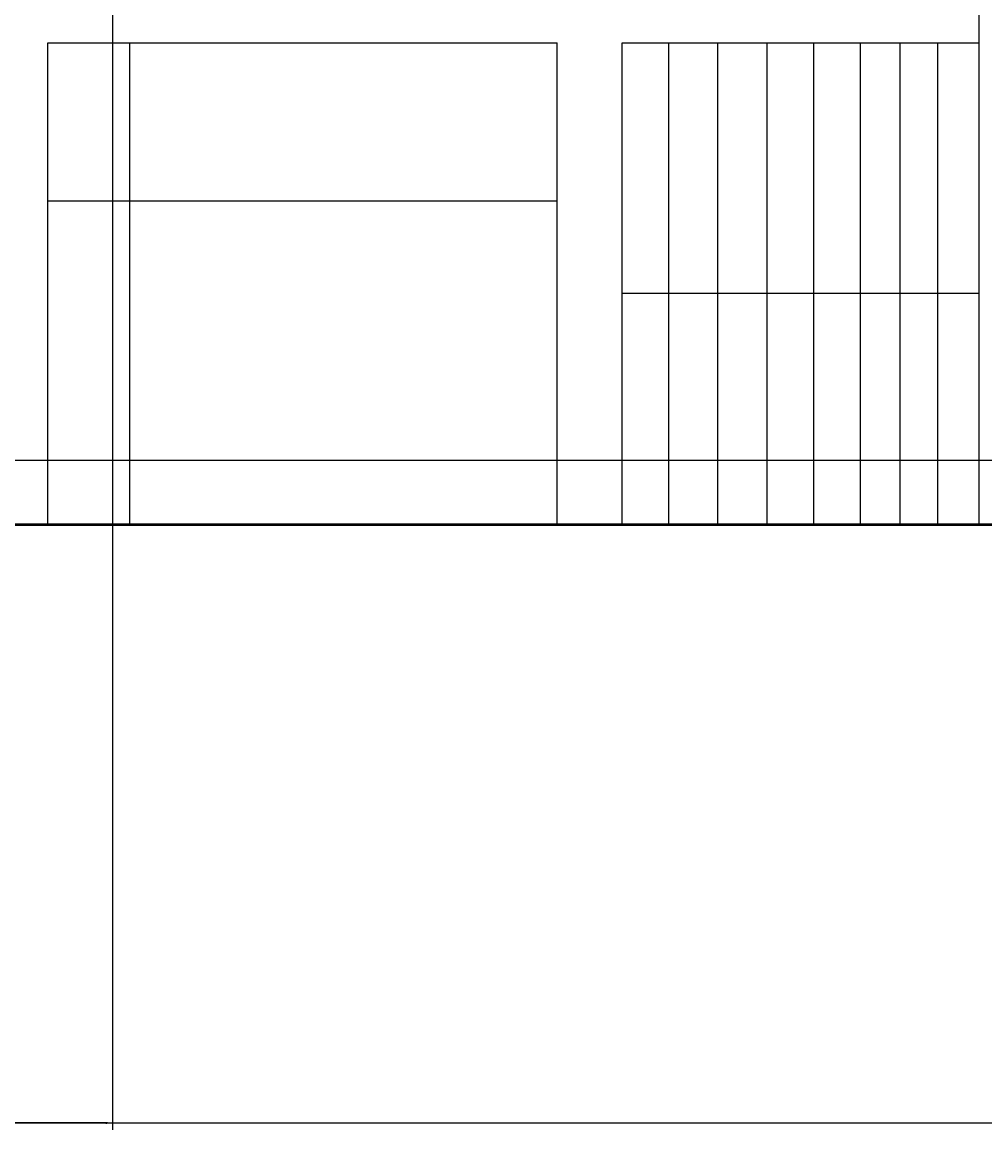
# Model space of a CAD drawing. Units: inches. Extents: x -117 to 121, y -77 to 40.
# Tile 6 of 45: x -48 to -23, y -77 to -48. Entities that reach past the tile are written whole.
import ezdxf

# ---------------------------------------------------------------- set-up
doc = ezdxf.new("R2010")
doc.units = ezdxf.units.IN
doc.header["$MEASUREMENT"] = 0
for name, color, linetype, lineweight in [('A-ANNO-DIMS', 2, 'Continuous', 18), ('A-ELEV', 7, 'Continuous', 25), ('A-ELEV-GRND', 7, 'Continuous', 50)]:
    doc.layers.add(name, color=color, linetype=linetype, lineweight=lineweight)
doc.styles.get("Standard").update_dxf_attribs({"font": 'arial.ttf'})
doc.dimstyles.get("Standard").update_dxf_attribs({"dimtxt": 0.18, "dimasz": 0.18, "dimexe": 0.18, "dimexo": 0.0625, "dimgap": 0.09, "dimtad": 0, "dimtih": 1, "dimtoh": 1, "dimdec": 4, "dimzin": 0, "dimdsep": 46, "dimtxsty": 'Standard', "dimcen": 0.09, "dimadec": 0, "dimazin": 0, "dimtfac": 1, "dimtdec": 4, "dimtofl": 0, "dimtmove": 0, "dimatfit": 3, "dimfxl": 1, "dimtolj": 1, "dimtzin": 0, "dimarcsym": 0})

# ---------------------------------------------------------------- blocks, each defined once
blk = doc.blocks.new('*D7')
at = {"layer": 'A-ANNO-DIMS', "color": 0, "lineweight": -2, "transparency": 16777216}
for p, q in [((-77.763, -61.431), (-77.763, -77.193)), ((90.549, -61.438), (90.549, -77.193)), ((-77.583, -77.013), (6.008, -77.013)), ((90.369, -77.013), (6.778, -77.013))]:
    blk.add_line(p, q, dxfattribs=at)
at = {"layer": 'A-ANNO-DIMS', "color": 0, "transparency": 16777216}
for points in [[(-77.583, -76.983), (-77.583, -77.043), (-77.763, -77.013)], [(90.369, -76.983), (90.369, -77.043), (90.549, -77.013)]]:
    blk.add_solid(points, dxfattribs=at)
at = {"layer": 'Defpoints', "color": 0, "transparency": 16777216}
for p in [(-77.763, -61.369), (90.549, -61.376), (90.549, -77.013)]:
    blk.add_point(p, dxfattribs=at)
at = {"layer": 'A-ANNO-DIMS', "color": 0, "transparency": 16777216, "insert": (6.393, -77.013), "char_height": 0.18, "attachment_point": 5}
blk.add_mtext('\\A1;168.3', dxfattribs=at)
blk = doc.blocks.new('*D13')
at = {"layer": 'A-ANNO-DIMS', "color": 0, "lineweight": -2, "transparency": 16777216}
for p, q in [((-2.663, 27.063), (-117.024, 27.063)), ((-116.844, 26.883), (-116.844, -16.974)), ((-116.844, -61.196), (-116.844, -17.338)), ((-106.096, -61.376), (-117.024, -61.376))]:
    blk.add_line(p, q, dxfattribs=at)
at = {"layer": 'A-ANNO-DIMS', "color": 0, "transparency": 16777216}
for points in [[(-116.874, 26.883), (-116.814, 26.883), (-116.844, 27.063)], [(-116.874, -61.196), (-116.814, -61.196), (-116.844, -61.376)]]:
    blk.add_solid(points, dxfattribs=at)
at = {"layer": 'Defpoints', "color": 0, "transparency": 16777216}
for p in [(-2.6, 27.063), (-116.844, -61.376), (-106.034, -61.376)]:
    blk.add_point(p, dxfattribs=at)
at = {"layer": 'A-ANNO-DIMS', "color": 0, "transparency": 16777216, "insert": (-116.844, -17.156), "char_height": 0.18, "attachment_point": 5}
blk.add_mtext('\\A1;88.44', dxfattribs=at)
blk = doc.blocks.new('*D37')
at = {"layer": 'A-ANNO-DIMS', "color": 0, "lineweight": -2, "transparency": 16777216}
for p, q in [((-3.912, -45.613), (-117.024, -45.613)), ((-116.844, -45.793), (-116.844, -52.47)), ((-116.844, -59.512), (-116.844, -52.834)), ((-3.912, -59.692), (-117.024, -59.692))]:
    blk.add_line(p, q, dxfattribs=at)
at = {"layer": 'A-ANNO-DIMS', "color": 0, "transparency": 16777216}
for points in [[(-116.874, -45.793), (-116.814, -45.793), (-116.844, -45.613)], [(-116.874, -59.512), (-116.814, -59.512), (-116.844, -59.692)]]:
    blk.add_solid(points, dxfattribs=at)
at = {"layer": 'Defpoints', "color": 0, "transparency": 16777216}
for p in [(-116.844, -45.613), (-3.85, -45.613), (-3.85, -59.692)]:
    blk.add_point(p, dxfattribs=at)
at = {"layer": 'A-ANNO-DIMS', "color": 0, "transparency": 16777216, "insert": (-116.844, -52.652), "char_height": 0.18, "attachment_point": 5}
blk.add_mtext('\\A1;14.079', dxfattribs=at)
blk = doc.blocks.new('*D48')
at = {"layer": 'A-ANNO-DIMS', "color": 0, "lineweight": -2, "transparency": 16777216}
for p, q in [((-65.167, -39.778), (-65.167, -77.193)), ((-45.533, -39.778), (-45.533, -77.193)), ((-64.987, -77.013), (-55.805, -77.013)), ((-45.713, -77.013), (-54.895, -77.013))]:
    blk.add_line(p, q, dxfattribs=at)
at = {"layer": 'A-ANNO-DIMS', "color": 0, "transparency": 16777216}
for points in [[(-64.987, -76.983), (-64.987, -77.043), (-65.167, -77.013)], [(-45.713, -76.983), (-45.713, -77.043), (-45.533, -77.013)]]:
    blk.add_solid(points, dxfattribs=at)
at = {"layer": 'Defpoints', "color": 0, "transparency": 16777216}
for p in [(-65.167, -39.716), (-45.533, -39.716), (-45.533, -77.013)]:
    blk.add_point(p, dxfattribs=at)
at = {"layer": 'A-ANNO-DIMS', "color": 0, "transparency": 16777216, "insert": (-55.35, -77.013), "char_height": 0.18, "attachment_point": 5}
blk.add_mtext('\\A1;19.634', dxfattribs=at)

msp = doc.modelspace()

# ---------------------------------------------------------------- linework, layer by layer
at = {"layer": 'A-ELEV'}
for p, q in [((-22.8601, -61.3756), (-22.8601, -31.9617)), ((-47.2265, -61.3756), (-47.2265, -48.7698)), ((-47.2265, -48.7698), (-33.8996, -48.7698)), ((-45.0735, -61.3756), (-45.0735, -48.7698)), ((-33.8996, -61.3756), (-33.8996, -48.7698)), ((-32.195, -61.3756), (-32.195, -48.7698)), ((-32.195, -48.7698), (-22.8601, -48.7698)), ((-30.9878, -48.7698), (-30.9878, -61.3756)), ((-29.7033, -48.7698), (-29.7033, -61.3756)), ((-28.4189, -48.7698), (-28.4189, -61.3756)), ((-27.1956, -48.7698), (-27.1956, -61.3756)), ((-25.9723, -48.7698), (-25.9723, -61.3756)), ((-24.9326, -48.7698), (-24.9326, -61.3756)), ((-23.9539, -48.7698), (-23.9539, -61.3756)), ((-47.2265, -52.905), (-33.8996, -52.905)), ((-32.195, -55.3185), (-22.8601, -55.3185))]:
    msp.add_line(p, q, dxfattribs=at)
at = {"layer": 'A-ELEV-GRND'}
msp.add_line((90.5486, -61.3756), (-87.9273, -61.3756), dxfattribs=at)

# ---------------------------------------------------------------- dimensions: what is measured, and where the dimension line sits
at = {"layer": 'A-ANNO-DIMS'}
for base, p1, p2, override, picture, middle in [((-116.8438, -61.3756), (-2.6001, 27.0634), (-106.0338, -61.3756), {"dimdec": 2, "dimlfac": 1, "dimrnd": 0, "dimzin": 0, "dimdsep": 46, "dimlunit": 2}, '*D13', (-116.8438, -17.1561)), ((-116.843772, -45.612514), (-3.849514, -59.692012), (-3.849514, -45.612514), {"dimdec": 3, "dimlfac": 1, "dimrnd": 0, "dimzin": 0, "dimdsep": 46, "dimlunit": 2}, '*D37', (-116.843772, -52.652263))]:
    dim = msp.add_linear_dim(base=base, p1=p1, p2=p2, angle=90, dimstyle='Standard', override=override, dxfattribs=at)
    dim.commit()
    dim.dimension.update_dxf_attribs({"geometry": picture, "text_midpoint": middle})
for base, p1, p2, override, picture, middle in [((-45.5331, -77.0135), (-65.1673, -39.716), (-45.5331, -39.716), {"dimdec": 3, "dimlfac": 1, "dimrnd": 0, "dimzin": 0, "dimdsep": 46, "dimlunit": 2}, '*D48', (-55.3502, -77.0135)), ((90.5486, -77.0135), (-77.7631, -61.3689), (90.5486, -61.3756), {"dimdec": 1, "dimlfac": 1, "dimrnd": 0, "dimzin": 0, "dimdsep": 46, "dimlunit": 2}, '*D7', (6.3928, -77.0135))]:
    dim = msp.add_linear_dim(base=base, p1=p1, p2=p2, dimstyle='Standard', override=override, dxfattribs=at)
    dim.commit()
    dim.dimension.update_dxf_attribs({"geometry": picture, "text_midpoint": middle})

doc.saveas('drawing.dxf')
